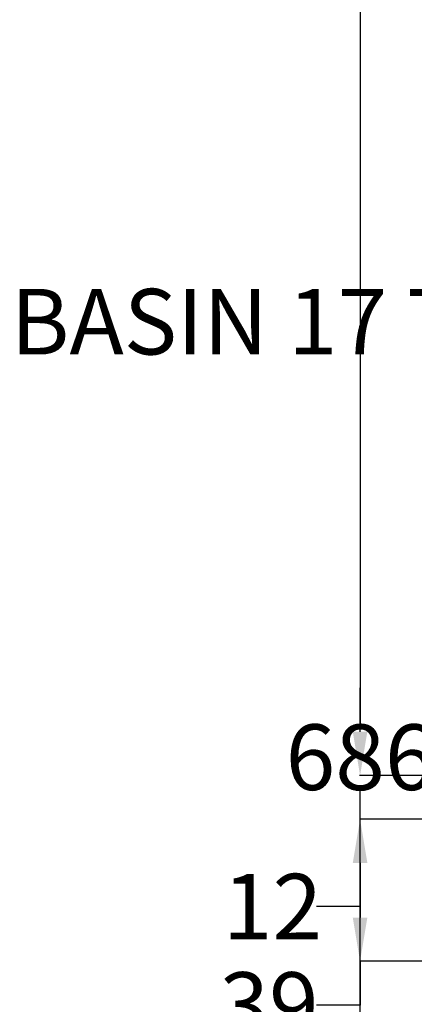
# Model space of a CAD drawing. Units: inches. Extents: x -230 to 384, y -962 to -183.
# Tile 2 of 6: x -230 to -121, y -640 to -370. Entities that reach past the tile are written whole.
import ezdxf

# ---------------------------------------------------------------- set-up
doc = ezdxf.new("R2010")
doc.units = ezdxf.units.IN
doc.layers.add('A-ANNO-DIMS', color=2, linetype='Continuous', lineweight=18)
doc.styles.get("Standard").update_dxf_attribs({"font": 'arial.ttf'})
doc.dimstyles.get("Standard").update_dxf_attribs({"dimtxt": 18, "dimasz": 12, "dimexe": 0.18, "dimexo": 0.0625, "dimgap": 0.09, "dimtad": 0, "dimtih": 1, "dimtoh": 1, "dimdec": 0, "dimzin": 0, "dimdsep": 46, "dimlunit": 3, "dimtxsty": 'Standard', "dimcen": 0.09, "dimadec": 0, "dimazin": 0, "dimtfac": 1, "dimtdec": 0, "dimtofl": 0, "dimtmove": 0, "dimatfit": 3, "dimfxl": 1, "dimtolj": 1, "dimtzin": 0, "dimarcsym": 0})

# ---------------------------------------------------------------- blocks, each defined once
blk = doc.blocks.new('*D20')
at = {"layer": 'A-ANNO-DIMS', "color": 0, "lineweight": -2, "transparency": 16777216}
for p, q in [((-43.76, -450.32), (-43.76, -452.95)), ((-26.97, -450.32), (-26.97, -452.95)), ((-55.76, -452.77), (-67.76, -452.77)), ((-14.97, -452.77), (-2.97, -452.77))]:
    blk.add_line(p, q, dxfattribs=at)
at = {"layer": 'A-ANNO-DIMS', "color": 0, "transparency": 16777216}
for points in [[(-55.76, -450.77), (-55.76, -454.77), (-43.76, -452.77)], [(-14.97, -450.77), (-14.97, -454.77), (-26.97, -452.77)]]:
    blk.add_solid(points, dxfattribs=at)
at = {"layer": 'Defpoints', "color": 0, "transparency": 16777216}
for p in [(-43.76, -450.25), (-26.97, -450.25), (-43.76, -452.77)]:
    blk.add_point(p, dxfattribs=at)
at = {"layer": 'A-ANNO-DIMS', "color": 0, "transparency": 16777216, "insert": (-152.48, -452.77), "char_height": 18, "attachment_point": 5}
blk.add_mtext('\\A1;BASIN 17 TYP.', dxfattribs=at)
blk = doc.blocks.new('*D33')
at = {"layer": 'A-ANNO-DIMS', "color": 0, "lineweight": -2, "transparency": 16777216}
for p, q in [((-101.66, -229.25), (-136.23, -229.25)), ((-136.05, -241.25), (-136.05, -562.97)), ((-136.05, -903.25), (-136.05, -581.53)), ((-101.66, -915.25), (-136.23, -915.25))]:
    blk.add_line(p, q, dxfattribs=at)
at = {"layer": 'A-ANNO-DIMS', "color": 0, "transparency": 16777216}
for points in [[(-138.05, -241.25), (-134.05, -241.25), (-136.05, -229.25)], [(-138.05, -903.25), (-134.05, -903.25), (-136.05, -915.25)]]:
    blk.add_solid(points, dxfattribs=at)
at = {"layer": 'Defpoints', "color": 0, "transparency": 16777216}
for p in [(-101.6, -229.25), (-136.05, -915.25), (-101.6, -915.25)]:
    blk.add_point(p, dxfattribs=at)
at = {"layer": 'A-ANNO-DIMS', "color": 0, "transparency": 16777216, "insert": (-136.05, -572.25), "char_height": 18, "attachment_point": 5}
blk.add_mtext('\\A1;686', dxfattribs=at)
blk = doc.blocks.new('*D39')
at = {"layer": 'A-ANNO-DIMS', "color": 0, "lineweight": -2, "transparency": 16777216}
for p, q in [((-56.66, -589.25), (-136.23, -589.25)), ((-136.05, -601.25), (-136.05, -616.25)), ((-56.66, -628.25), (-136.23, -628.25)), ((-136.05, -628.25), (-136.05, -640.25)), ((-136.05, -640.25), (-148.05, -640.25))]:
    blk.add_line(p, q, dxfattribs=at)
at = {"layer": 'A-ANNO-DIMS', "color": 0, "transparency": 16777216}
for points in [[(-138.05, -601.25), (-134.05, -601.25), (-136.05, -589.25)], [(-138.05, -616.25), (-134.05, -616.25), (-136.05, -628.25)]]:
    blk.add_solid(points, dxfattribs=at)
at = {"layer": 'Defpoints', "color": 0, "transparency": 16777216}
for p in [(-56.6, -589.25), (-136.05, -628.25), (-56.6, -628.25)]:
    blk.add_point(p, dxfattribs=at)
at = {"layer": 'A-ANNO-DIMS', "color": 0, "transparency": 16777216, "insert": (-161.05, -640.25), "char_height": 18, "attachment_point": 5}
blk.add_mtext('\\A1;39', dxfattribs=at)
blk = doc.blocks.new('*D48')
at = {"layer": 'A-ANNO-DIMS', "color": 0, "lineweight": -2, "transparency": 16777216}
for p, q in [((-136.05, -565.25), (-136.05, -553.25)), ((-56.66, -577.25), (-136.23, -577.25)), ((-56.66, -589.25), (-136.23, -589.25)), ((-136.05, -601.25), (-136.05, -613.25)), ((-136.05, -613.25), (-148.05, -613.25))]:
    blk.add_line(p, q, dxfattribs=at)
at = {"layer": 'A-ANNO-DIMS', "color": 0, "transparency": 16777216}
for points in [[(-138.05, -565.25), (-134.05, -565.25), (-136.05, -577.25)], [(-138.05, -601.25), (-134.05, -601.25), (-136.05, -589.25)]]:
    blk.add_solid(points, dxfattribs=at)
at = {"layer": 'Defpoints', "color": 0, "transparency": 16777216}
for p in [(-56.6, -577.25), (-136.05, -589.25), (-56.6, -589.25)]:
    blk.add_point(p, dxfattribs=at)
at = {"layer": 'A-ANNO-DIMS', "color": 0, "transparency": 16777216, "insert": (-160.09, -613.25), "char_height": 18, "attachment_point": 5}
blk.add_mtext('\\A1;12', dxfattribs=at)

msp = doc.modelspace()

# ---------------------------------------------------------------- dimensions: what is measured, and where the dimension line sits
at = {"layer": 'A-ANNO-DIMS'}
for base, p1, p2, picture, middle in [((-136.05, -915.25), (-101.6, -229.25), (-101.6, -915.25), '*D33', (-136.05, -572.25)), ((-136.05, -589.25), (-56.6, -577.25), (-56.6, -589.25), '*D48', (-160.09, -613.25)), ((-136.05, -628.25), (-56.6, -589.25), (-56.6, -628.25), '*D39', (-161.05, -640.25))]:
    dim = msp.add_linear_dim(base=base, p1=p1, p2=p2, angle=90, dimstyle='Standard', override={"dimdec": 0, "dimlfac": 1, "dimrnd": 0, "dimzin": 0, "dimdsep": 46, "dimlunit": 2}, dxfattribs=at)
    dim.commit()
    dim.dimension.update_dxf_attribs({"geometry": picture, "text_midpoint": middle})
dim = msp.add_linear_dim(base=(-43.76, -452.77), p1=(-26.97, -450.25), p2=(-43.76, -450.25), angle=180, text='BASIN <> TYP.', dimstyle='Standard', override={"dimdec": 0, "dimlfac": 1, "dimrnd": 0, "dimzin": 0, "dimdsep": 46, "dimlunit": 2}, dxfattribs=at)
dim.commit()
dim.dimension.update_dxf_attribs({"geometry": '*D20', "text_midpoint": (-152.48, -452.77)})

doc.saveas('drawing.dxf')
